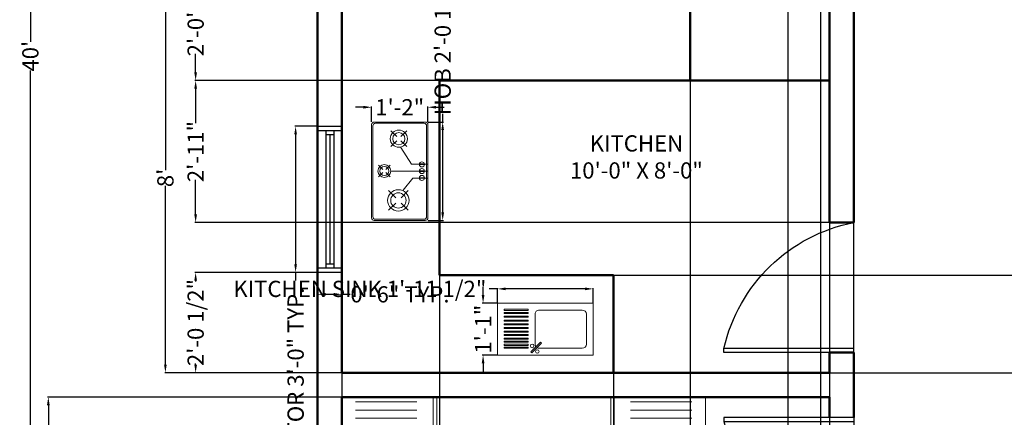
# Model space of a CAD drawing. Units: inches. Extents: x 2663 to 3147, y 140 to 736.
# Tile 2 of 6: x 2663 to 2905, y 327 to 425. Entities that reach past the tile are written whole.
import ezdxf

# ---------------------------------------------------------------- set-up
doc = ezdxf.new("R2010")
doc.units = ezdxf.units.IN
doc.header["$MEASUREMENT"] = 0
for name, color, linetype, lineweight in [('A-ANNO-DIMS', 2, 'Continuous', 18), ('A-AREA-IDEN', 3, 'Continuous', 25), ('A-DOOR', 3, 'Continuous', 25), ('A-FLOR-FIXT', 9, 'Continuous', 18), ('A-FURN', 8, 'Continuous', 18), ('A-GLAZ', 4, 'Continuous', 25), ('A-WALL', 7, 'Continuous', 50)]:
    doc.layers.add(name, color=color, linetype=linetype, lineweight=lineweight)
doc.styles.get("Standard").update_dxf_attribs({"font": 'arial.ttf'})
doc.dimstyles.get("Standard").update_dxf_attribs({"dimtxt": 4, "dimasz": 2, "dimexe": 0.18, "dimexo": 0.0625, "dimgap": 0.09, "dimtad": 0, "dimdec": 0, "dimzin": 0, "dimdsep": 46, "dimlunit": 4, "dimtxsty": 'Standard', "dimcen": 0.09, "dimadec": 0, "dimazin": 0, "dimtfac": 1, "dimtdec": 0, "dimtofl": 0, "dimtmove": 0, "dimatfit": 3, "dimfxl": 1, "dimtolj": 1, "dimtzin": 0, "dimarcsym": 0})

# ---------------------------------------------------------------- blocks, each defined once
blk = doc.blocks.new('*D4')
at = {"layer": 'A-ANNO-DIMS', "color": 0, "lineweight": -2, "transparency": 16777216}
for p, q in [((2742.1, 332.32), (2669.73, 332.32)), ((2669.91, 330.32), (2669.91, 264.1)), ((2669.91, 184.32), (2669.91, 250.55)), ((2742.1, 182.32), (2669.73, 182.32))]:
    blk.add_line(p, q, dxfattribs=at)
at = {"layer": 'A-ANNO-DIMS', "color": 0, "transparency": 16777216}
for points in [[(2669.57, 330.32), (2670.24, 330.32), (2669.91, 332.32)], [(2669.57, 184.32), (2670.24, 184.32), (2669.91, 182.32)]]:
    blk.add_solid(points, dxfattribs=at)
at = {"layer": 'Defpoints', "color": 0, "transparency": 16777216}
for p in [(2669.91, 332.32), (2742.16, 332.32), (2742.16, 182.32)]:
    blk.add_point(p, dxfattribs=at)
at = {"layer": 'A-ANNO-DIMS', "color": 0, "transparency": 16777216, "insert": (2669.91, 257.32), "char_height": 4, "attachment_point": 5, "rotation": 90}
blk.add_mtext('\\A1;12\'-6"', dxfattribs=at)
blk = doc.blocks.new('*D5')
at = {"layer": 'A-ANNO-DIMS', "color": 0, "lineweight": -2, "transparency": 16777216}
for p, q in [((2742.1, 434.32), (2698.54, 434.32)), ((2698.72, 432.32), (2698.72, 388.26)), ((2698.72, 340.32), (2698.72, 384.39)), ((2742.1, 338.32), (2698.54, 338.32))]:
    blk.add_line(p, q, dxfattribs=at)
at = {"layer": 'A-ANNO-DIMS', "color": 0, "transparency": 16777216}
for points in [[(2698.38, 432.32), (2699.05, 432.32), (2698.72, 434.32)], [(2698.38, 340.32), (2699.05, 340.32), (2698.72, 338.32)]]:
    blk.add_solid(points, dxfattribs=at)
at = {"layer": 'Defpoints', "color": 0, "transparency": 16777216}
for p in [(2698.72, 434.32), (2742.16, 434.32), (2742.16, 338.32)]:
    blk.add_point(p, dxfattribs=at)
at = {"layer": 'A-ANNO-DIMS', "color": 0, "transparency": 16777216, "insert": (2698.72, 386.32), "char_height": 4, "attachment_point": 5, "rotation": 90}
blk.add_mtext("\\A1;8'", dxfattribs=at)
blk = doc.blocks.new('FGCHBJK')
for p, q in [((3315.88, 342.07), (3315.88, 348.07)), ((3315.88, 348.07), (3351.88, 348.07)), ((3316.88, 342.07), (3316.88, 348.07)), ((3350.88, 348.07), (3350.88, 342.07)), ((3351.88, 348.07), (3351.88, 342.07)), ((3316.88, 346.07), (3350.88, 346.07)), ((3316.88, 344.07), (3350.88, 344.07)), ((3317.88, 344.07), (3317.88, 346.07)), ((3317.88, 345.07), (3349.88, 345.07)), ((3349.88, 346.07), (3349.88, 344.07)), ((3351.88, 342.07), (3315.88, 342.07))]:
    blk.add_line(p, q)
blk = doc.blocks.new('A$C34930FF8')
at = {"ltscale": 0.05}
for p, q in [((0, 2252.4), (0, 16.8)), ((600, 2252.4), (0, 2252.4)), ((185.4, 1513), (185.4, 1521.5)), ((237.7, 1513), (237.7, 1521.5)), ((227.1, 1479.2), (233.2, 1485.2)), ((436.7, 1513), (436.7, 1504.4)), ((482.5, 1513), (482.5, 1504.4)), ((263.6, 1441.7), (269.7, 1447.7)), ((398.2, 1303.6), (392.1, 1297.6)), ((185.4, 1229.1), (185.4, 1237.7)), ((237.7, 1229.1), (237.7, 1237.7)), ((434.8, 1266.1), (428.7, 1260.1)), ((436.7, 1228.2), (436.7, 1219.7)), ((482.5, 1228.2), (482.5, 1219.7)), ((209.5, 1150.1), (214.1, 1157.3)), ((253.5, 1121.8), (258.1, 1129)), ((415.3, 1017.6), (410.6, 1010.5)), ((459.3, 989.3), (454.7, 982.1)), ((482.5, 894.9), (482.5, 886.3)), ((237.7, 775.3), (237.7, 783.9)), ((436.7, 775.3), (436.7, 766.8)), ((482.5, 775.3), (482.5, 766.8)), ((600, 16.8), (0, 16.8))]:
    blk.add_line(p, q, dxfattribs=at)
for p, q in [((580, 1690.9), (580, 2252.4)), ((600, 1669.3), (600, 2269.3)), ((30, 1790.9), (30, 2169.3)), ((80, 1790.9), (80, 2169.3)), ((130, 1790.9), (130, 2169.3)), ((180, 1790.9), (180, 2169.3)), ((230, 1790.9), (230, 2169.3)), ((280, 1790.9), (280, 2169.3)), ((330, 1790.9), (330, 2169.3)), ((380, 1790.9), (380, 2169.3)), ((430, 1790.9), (430, 2169.3)), ((480, 1790.9), (480, 2169.3)), ((530, 1790.9), (530, 2169.3)), ((580, 1690.9), (0, 1690.9)), ((600, 1669.3), (0, 1669.3)), ((335.4, 1666.1), (335.4, 603.1)), ((600, 1603.3), (620, 1603.3)), ((600, 1018.7), (600, 1603.3)), ((620, 1603.3), (620, 1018.7)), ((237.7, 1521.5), (185.4, 1521.5)), ((482.5, 1513), (185.4, 1513)), ((434.8, 1266.1), (227.4, 1478.9)), ((269.7, 1447.7), (233.2, 1485.2)), ((436.7, 1504.4), (482.5, 1504.4)), ((428.7, 1260.1), (392.1, 1297.6)), ((237.7, 1237.7), (185.4, 1237.7)), ((482.5, 1228.2), (185.4, 1228.2)), ((436.7, 1219.7), (482.5, 1219.7)), ((600, 1233.4), (580, 1233.4)), ((580, 1233.4), (580, 648.7)), ((600, 648.7), (600, 1233.4)), ((258.1, 1129), (214.1, 1157.3)), ((459.3, 989.3), (209.5, 1150.1)), ((454.7, 982.1), (410.6, 1010.5)), ((620, 1018.7), (600, 1018.7)), ((482.5, 894.9), (185.4, 894.9)), ((436.7, 886.3), (482.5, 886.3)), ((237.7, 783.9), (185.4, 783.9)), ((482.5, 775.3), (185.4, 775.3)), ((436.7, 766.8), (482.5, 766.8)), ((580, 648.7), (600, 648.7)), ((600, 600), (0, 600)), ((580, 578.3), (0, 578.3)), ((580, 578.3), (580, 16.8)), ((600, 600), (600, 0)), ((30, 478.3), (30, 100)), ((80, 478.3), (80, 100)), ((130, 478.3), (130, 100)), ((180, 478.3), (180, 100)), ((230, 478.3), (230, 100)), ((280, 478.3), (280, 100)), ((330, 478.3), (330, 100)), ((380, 478.3), (380, 100)), ((430, 478.3), (430, 100)), ((480, 478.3), (480, 100)), ((530, 478.3), (530, 100))]:
    blk.add_line(p, q)
blk = doc.blocks.new('DXFGVHBJKL')
for p, q in [((2908.16, 532.32), (2907.16, 532.32)), ((2907.16, 532.32), (2907.16, 500.32)), ((2908.16, 500.32), (2908.16, 532.32)), ((2908.16, 500.32), (2876.16, 500.32))]:
    blk.add_line(p, q)
blk.add_arc((2916.21, 492.54), 40.8, 102.812, 169.0067)
blk = doc.blocks.new('A$C67F5712B')
for p, q in [((0, 415), (0, 20)), ((10, 405), (10, 30)), ((20, 435), (742, 435)), ((30, 425), (732, 425)), ((336.9, 382.4), (370.3, 349)), ((428.4, 382.4), (394.9, 349)), ((752, 405), (752, 30)), ((762, 415), (762, 20)), ((336.9, 291), (370.3, 324.4)), ((428.4, 291), (394.9, 324.4)), ((79.2, 304.2), (134.9, 248.4)), ((231.6, 304.2), (175.9, 248.4)), ((381, 65.3), (381, 287.1)), ((572, 285.4), (616.6, 240.8)), ((694, 285.4), (649.4, 240.8)), ((79.2, 151.7), (134.9, 207.5)), ((231.6, 151.7), (175.9, 207.5)), ((234.5, 189.9), (328.8, 115.2)), ((435.3, 127.1), (564.3, 209.7)), ((572, 163.4), (616.6, 208)), ((694, 163.4), (649.4, 208)), ((328.8, 65.3), (328.8, 115.2)), ((435.3, 65.3), (435.3, 127.1)), ((30, 10), (732, 10)), ((327.2, 61), (331, 61)), ((327.2, 30.4), (327.2, 61)), ((331, 30.4), (327.2, 30.4)), ((328.8, 0), (328.8, 25.9)), ((331, 61), (331, 30.4)), ((379.4, 61), (383.2, 61)), ((379.4, 30.4), (379.4, 61)), ((383.2, 30.4), (379.4, 30.4)), ((381, 0), (381, 25.9)), ((383.2, 61), (383.2, 30.4)), ((433.7, 61), (437.5, 61)), ((433.7, 30.4), (433.7, 61)), ((437.5, 30.4), (433.7, 30.4)), ((435.3, 0), (435.3, 25.9)), ((437.5, 61), (437.5, 30.4)), ((20, 0), (742, 0))]:
    blk.add_line(p, q)
for centre, radius in [((382.6, 336.7), 49.7), ((155.4, 228), 82.8), ((382.6, 336.7), 35.4), ((155.4, 228), 59), ((633, 224.4), 66.2), ((633, 224.4), 47.2), ((329.2, 45.6), 19.7), ((382.6, 45.6), 19.7), ((434.4, 45.6), 19.7)]:
    blk.add_circle(centre, radius)
for centre, start, end in [((20, 415), 90, 180), ((30, 405), 90, 180), ((732, 405), 0, 90), ((742, 415), 0, 90), ((20, 20), 180, 270), ((30, 30), 180, 270), ((732, 30), 270, 0), ((742, 20), 270, 0)]:
    blk.add_arc(centre, 20, start, end)
blk = doc.blocks.new('A$C49617FB3')
for p, q in [((0, 0), (0, 380.2)), ((0, 380.2), (700.3, 380.2)), ((378.5, 293.7), (448.3, 363.5)), ((448.3, 363.5), (456.5, 355.2)), ((700.3, 380.2), (700.3, 0)), ((50, 80), (50, 300.1)), ((80, 330.1), (395.2, 330.1)), ((386.7, 285.4), (378.5, 293.7)), ((456.5, 355.2), (386.7, 285.4)), ((425.2, 80), (425.2, 300.1)), ((475.2, 322.3), (475.2, 330.1)), ((475.2, 330.1), (650.7, 330.1)), ((475.2, 330.1), (650.3, 330.1)), ((650.7, 322.3), (475.2, 322.3)), ((475.2, 301), (475.2, 308.8)), ((475.2, 308.8), (650.7, 308.8)), ((650.7, 301), (475.2, 301)), ((650.7, 330.1), (650.7, 322.3)), ((650.7, 308.8), (650.7, 301)), ((475.2, 278.2), (475.2, 286)), ((475.2, 286), (650.7, 286)), ((650.7, 278.2), (475.2, 278.2)), ((475.2, 255.4), (475.2, 263.3)), ((475.2, 263.3), (650.7, 263.3)), ((650.7, 255.4), (475.2, 255.4)), ((475.2, 229.8), (475.2, 237.6)), ((475.2, 237.6), (650.7, 237.6)), ((650.7, 229.8), (475.2, 229.8)), ((650.7, 286), (650.7, 278.2)), ((650.7, 263.3), (650.7, 255.4)), ((650.7, 237.6), (650.7, 229.8)), ((475.2, 204.2), (475.2, 212)), ((475.2, 212), (650.7, 212)), ((650.7, 204.2), (475.2, 204.2)), ((475.2, 178.6), (475.2, 186.4)), ((475.2, 186.4), (650.7, 186.4)), ((650.7, 178.6), (475.2, 178.6)), ((475.2, 151.5), (475.2, 159.3)), ((475.2, 159.3), (650.7, 159.3)), ((650.7, 151.5), (475.2, 151.5)), ((650.7, 212), (650.7, 204.2)), ((650.7, 186.4), (650.7, 178.6)), ((650.7, 159.3), (650.7, 151.5)), ((475.2, 124.5), (475.2, 132.3)), ((475.2, 132.3), (650.7, 132.3)), ((650.7, 124.5), (475.2, 124.5)), ((475.2, 94.6), (475.2, 102.4)), ((475.2, 102.4), (650.7, 102.4)), ((650.7, 94.6), (475.2, 94.6)), ((475.2, 67.5), (475.2, 75.4)), ((475.2, 75.4), (650.7, 75.4)), ((650.7, 132.3), (650.7, 124.5)), ((650.7, 102.4), (650.7, 94.6)), ((650.7, 75.4), (650.7, 67.5)), ((395.2, 50), (80, 50)), ((650.7, 67.5), (475.2, 67.5)), ((475.2, 44.8), (475.2, 52.6)), ((475.2, 52.6), (650.7, 52.6)), ((650.7, 44.8), (475.2, 44.8)), ((650.7, 52.6), (650.7, 44.8)), ((700.3, 0), (0, 0))]:
    blk.add_line(p, q)
for centre in [(408.3, 353.3), (446.1, 312.6)]:
    blk.add_circle(centre, 13)
for centre, start, end in [((80, 300.1), 90, 180), ((395.2, 300.1), 58.92551, 90), ((395.2, 300.1), 0, 36.55582), ((80, 80), 180, 270), ((395.2, 80), 270, 0)]:
    blk.add_arc(centre, 30, start, end)
blk = doc.blocks.new('*D37')
at = {"layer": 'A-ANNO-DIMS', "color": 0, "lineweight": -2, "transparency": 16777216}
for p, q in [((2736.1, 656.32), (2665.31, 656.32)), ((2665.49, 654.32), (2665.49, 419.89)), ((2665.49, 178.32), (2665.49, 412.76)), ((2736.1, 176.32), (2665.31, 176.32))]:
    blk.add_line(p, q, dxfattribs=at)
at = {"layer": 'A-ANNO-DIMS', "color": 0, "transparency": 16777216}
for points in [[(2665.15, 654.32), (2665.82, 654.32), (2665.49, 656.32)], [(2665.15, 178.32), (2665.82, 178.32), (2665.49, 176.32)]]:
    blk.add_solid(points, dxfattribs=at)
at = {"layer": 'Defpoints', "color": 0, "transparency": 16777216}
for p in [(2665.49, 656.32), (2736.16, 656.32), (2736.16, 176.32)]:
    blk.add_point(p, dxfattribs=at)
at = {"layer": 'A-ANNO-DIMS', "color": 0, "transparency": 16777216, "insert": (2665.49, 416.32), "char_height": 4, "attachment_point": 5, "rotation": 90}
blk.add_mtext("\\A1;40'", dxfattribs=at)
blk = doc.blocks.new('*D43')
at = {"layer": 'A-ANNO-DIMS', "color": 0, "lineweight": -2, "transparency": 16777216}
for p, q in [((2736.1, 399.04), (2730.58, 399.04)), ((2730.76, 397.04), (2730.76, 365.04)), ((2736.1, 363.04), (2730.58, 363.04)), ((2730.76, 363.04), (2730.76, 361.04))]:
    blk.add_line(p, q, dxfattribs=at)
at = {"layer": 'A-ANNO-DIMS', "color": 0, "transparency": 16777216}
for points in [[(2730.43, 397.04), (2731.09, 397.04), (2730.76, 399.04)], [(2730.43, 365.04), (2731.09, 365.04), (2730.76, 363.04)]]:
    blk.add_solid(points, dxfattribs=at)
at = {"layer": 'Defpoints', "color": 0, "transparency": 16777216}
for p in [(2736.16, 399.04), (2730.76, 363.04), (2736.16, 363.04)]:
    blk.add_point(p, dxfattribs=at)
at = {"layer": 'A-ANNO-DIMS', "color": 0, "transparency": 16777216, "insert": (2730.76, 330.34), "char_height": 4, "attachment_point": 5, "rotation": 90}
blk.add_mtext('\\A1;VENTILATOR 3\'-0" TYP.', dxfattribs=at)
blk = doc.blocks.new('*D44')
at = {"layer": 'A-ANNO-DIMS', "color": 0, "lineweight": -2, "transparency": 16777216}
for p, q in [((2736.16, 362.98), (2736.16, 357.46)), ((2742.16, 362.98), (2742.16, 357.46)), ((2738.16, 357.64), (2740.16, 357.64)), ((2742.16, 357.64), (2744.16, 357.64))]:
    blk.add_line(p, q, dxfattribs=at)
at = {"layer": 'A-ANNO-DIMS', "color": 0, "transparency": 16777216}
for points in [[(2738.16, 357.98), (2738.16, 357.31), (2736.16, 357.64)], [(2740.16, 357.98), (2740.16, 357.31), (2742.16, 357.64)]]:
    blk.add_solid(points, dxfattribs=at)
at = {"layer": 'Defpoints', "color": 0, "transparency": 16777216}
for p in [(2736.16, 363.04), (2742.16, 363.04), (2742.16, 357.64)]:
    blk.add_point(p, dxfattribs=at)
at = {"layer": 'A-ANNO-DIMS', "color": 0, "transparency": 16777216, "insert": (2756.44, 357.64), "char_height": 4, "attachment_point": 5}
blk.add_mtext('\\A1;0\'-6" TYP.', dxfattribs=at)
blk = doc.blocks.new('*D53')
at = {"layer": 'A-ANNO-DIMS', "color": 0, "lineweight": -2, "transparency": 16777216}
for p, q in [((2763.37, 400.1), (2767.13, 400.1)), ((2766.95, 400.1), (2766.95, 402.1)), ((2766.95, 377.83), (2766.95, 398.1)), ((2763.37, 375.83), (2767.13, 375.83))]:
    blk.add_line(p, q, dxfattribs=at)
at = {"layer": 'A-ANNO-DIMS', "color": 0, "transparency": 16777216}
for points in [[(2766.62, 398.1), (2767.29, 398.1), (2766.95, 400.1)], [(2766.62, 377.83), (2767.29, 377.83), (2766.95, 375.83)]]:
    blk.add_solid(points, dxfattribs=at)
at = {"layer": 'Defpoints', "color": 0, "transparency": 16777216}
for p in [(2763.31, 400.1), (2766.95, 400.1), (2763.31, 375.83)]:
    blk.add_point(p, dxfattribs=at)
at = {"layer": 'A-ANNO-DIMS', "color": 0, "transparency": 16777216, "insert": (2766.95, 418.89), "char_height": 4, "attachment_point": 5, "rotation": 90}
blk.add_mtext('\\A1;HOB 2\'-0 1/2"', dxfattribs=at)
blk = doc.blocks.new('*D54')
at = {"layer": 'A-ANNO-DIMS', "color": 0, "lineweight": -2, "transparency": 16777216}
for p, q in [((2747.46, 403.74), (2745.46, 403.74)), ((2749.46, 400.17), (2749.46, 403.92)), ((2763.31, 400.17), (2763.31, 403.92)), ((2765.31, 403.74), (2767.31, 403.74))]:
    blk.add_line(p, q, dxfattribs=at)
at = {"layer": 'A-ANNO-DIMS', "color": 0, "transparency": 16777216}
for points in [[(2747.46, 404.08), (2747.46, 403.41), (2749.46, 403.74)], [(2765.31, 404.08), (2765.31, 403.41), (2763.31, 403.74)]]:
    blk.add_solid(points, dxfattribs=at)
at = {"layer": 'Defpoints', "color": 0, "transparency": 16777216}
for p in [(2749.46, 403.74), (2749.46, 400.1), (2763.31, 400.1)]:
    blk.add_point(p, dxfattribs=at)
at = {"layer": 'A-ANNO-DIMS', "color": 0, "transparency": 16777216, "insert": (2756.38, 403.74), "char_height": 4, "attachment_point": 5}
blk.add_mtext('\\A1;1\'-2"', dxfattribs=at)
blk = doc.blocks.new('*D55')
at = {"layer": 'A-ANNO-DIMS', "color": 0, "lineweight": -2, "transparency": 16777216}
for p, q in [((2780.43, 358.98), (2778.43, 358.98)), ((2780.43, 355.51), (2780.43, 359.16)), ((2802, 358.98), (2782.43, 358.98)), ((2804, 355.51), (2804, 359.16))]:
    blk.add_line(p, q, dxfattribs=at)
at = {"layer": 'A-ANNO-DIMS', "color": 0, "transparency": 16777216}
for points in [[(2782.43, 359.32), (2782.43, 358.65), (2780.43, 358.98)], [(2802, 359.32), (2802, 358.65), (2804, 358.98)]]:
    blk.add_solid(points, dxfattribs=at)
at = {"layer": 'Defpoints', "color": 0, "transparency": 16777216}
for p in [(2780.43, 358.98), (2780.43, 355.45), (2804, 355.45)]:
    blk.add_point(p, dxfattribs=at)
at = {"layer": 'A-ANNO-DIMS', "color": 0, "transparency": 16777216, "insert": (2746.56, 358.98), "char_height": 4, "attachment_point": 5}
blk.add_mtext('\\A1;KITCHEN SINK 1\'-11 1/2"', dxfattribs=at)
blk = doc.blocks.new('*D56')
at = {"layer": 'A-ANNO-DIMS', "color": 0, "lineweight": -2, "transparency": 16777216}
for p, q in [((2776.89, 357.45), (2776.89, 359.45)), ((2780.36, 355.45), (2776.71, 355.45)), ((2780.36, 342.65), (2776.71, 342.65)), ((2776.89, 340.65), (2776.89, 338.65))]:
    blk.add_line(p, q, dxfattribs=at)
at = {"layer": 'A-ANNO-DIMS', "color": 0, "transparency": 16777216}
for points in [[(2776.56, 357.45), (2777.22, 357.45), (2776.89, 355.45)], [(2776.56, 340.65), (2777.22, 340.65), (2776.89, 342.65)]]:
    blk.add_solid(points, dxfattribs=at)
at = {"layer": 'Defpoints', "color": 0, "transparency": 16777216}
for p in [(2780.43, 355.45), (2776.89, 342.65), (2780.43, 342.65)]:
    blk.add_point(p, dxfattribs=at)
at = {"layer": 'A-ANNO-DIMS', "color": 0, "transparency": 16777216, "insert": (2776.89, 349.05), "char_height": 4, "attachment_point": 5, "rotation": 90}
blk.add_mtext('\\A1;1\'-1"', dxfattribs=at)
blk = doc.blocks.new('*D61')
at = {"layer": 'A-ANNO-DIMS', "color": 0, "lineweight": -2, "transparency": 16777216}
for p, q in [((2851.95, 276.84), (2851.95, 686.5)), ((2853.95, 686.32), (2857.98, 686.32)), ((2859.98, 276.84), (2859.98, 686.5)), ((2859.98, 686.32), (2861.98, 686.32))]:
    blk.add_line(p, q, dxfattribs=at)
at = {"layer": 'A-ANNO-DIMS', "color": 0, "transparency": 16777216}
for points in [[(2853.95, 686.66), (2853.95, 685.99), (2851.95, 686.32)], [(2857.98, 686.66), (2857.98, 685.99), (2859.98, 686.32)]]:
    blk.add_solid(points, dxfattribs=at)
at = {"layer": 'Defpoints', "color": 0, "transparency": 16777216}
for p in [(2859.98, 686.32), (2851.95, 276.78), (2859.98, 276.78)]:
    blk.add_point(p, dxfattribs=at)
at = {"layer": 'A-ANNO-DIMS', "color": 0, "transparency": 16777216, "insert": (2867.39, 686.32), "char_height": 4, "attachment_point": 5}
blk.add_mtext('\\A1;0\'-8"', dxfattribs=at)
blk = doc.blocks.new('*D73')
at = {"layer": 'A-ANNO-DIMS', "color": 0, "lineweight": -2, "transparency": 16777216}
for p, q in [((2742.1, 363.04), (2705.98, 363.04)), ((2706.16, 361.04), (2706.16, 360.78)), ((2706.16, 340.32), (2706.16, 340.58)), ((2742.1, 338.32), (2705.98, 338.32))]:
    blk.add_line(p, q, dxfattribs=at)
at = {"layer": 'A-ANNO-DIMS', "color": 0, "transparency": 16777216}
for points in [[(2705.83, 361.04), (2706.49, 361.04), (2706.16, 363.04)], [(2705.83, 340.32), (2706.49, 340.32), (2706.16, 338.32)]]:
    blk.add_solid(points, dxfattribs=at)
at = {"layer": 'Defpoints', "color": 0, "transparency": 16777216}
for p in [(2706.16, 363.04), (2742.16, 363.04), (2742.16, 338.32)]:
    blk.add_point(p, dxfattribs=at)
at = {"layer": 'A-ANNO-DIMS', "color": 0, "transparency": 16777216, "insert": (2706.16, 350.68), "char_height": 4, "attachment_point": 5, "rotation": 90}
blk.add_mtext('\\A1;2\'-0 1/2"', dxfattribs=at)
blk = doc.blocks.new('*D79')
at = {"layer": 'A-ANNO-DIMS', "color": 0, "lineweight": -2, "transparency": 16777216}
for p, q in [((2862.1, 410.32), (2705.98, 410.32)), ((2706.16, 408.32), (2706.16, 399.82)), ((2706.16, 377.32), (2706.16, 385.83)), ((2862.1, 375.32), (2705.98, 375.32))]:
    blk.add_line(p, q, dxfattribs=at)
at = {"layer": 'A-ANNO-DIMS', "color": 0, "transparency": 16777216}
for points in [[(2705.83, 408.32), (2706.49, 408.32), (2706.16, 410.32)], [(2705.83, 377.32), (2706.49, 377.32), (2706.16, 375.32)]]:
    blk.add_solid(points, dxfattribs=at)
at = {"layer": 'Defpoints', "color": 0, "transparency": 16777216}
for p in [(2706.16, 410.32), (2862.16, 410.32), (2862.16, 375.32)]:
    blk.add_point(p, dxfattribs=at)
at = {"layer": 'A-ANNO-DIMS', "color": 0, "transparency": 16777216, "insert": (2706.16, 392.82), "char_height": 4, "attachment_point": 5, "rotation": 90}
blk.add_mtext('\\A1;2\'-11"', dxfattribs=at)
blk = doc.blocks.new('*D80')
at = {"layer": 'A-ANNO-DIMS', "color": 0, "lineweight": -2, "transparency": 16777216}
for p, q in [((2862.1, 434.32), (2705.98, 434.32)), ((2706.16, 432.32), (2706.16, 427.76)), ((2706.16, 412.32), (2706.16, 416.88)), ((2862.1, 410.32), (2705.98, 410.32))]:
    blk.add_line(p, q, dxfattribs=at)
at = {"layer": 'A-ANNO-DIMS', "color": 0, "transparency": 16777216}
for points in [[(2705.83, 432.32), (2706.49, 432.32), (2706.16, 434.32)], [(2705.83, 412.32), (2706.49, 412.32), (2706.16, 410.32)]]:
    blk.add_solid(points, dxfattribs=at)
at = {"layer": 'Defpoints', "color": 0, "transparency": 16777216}
for p in [(2706.16, 434.32), (2862.16, 434.32), (2862.16, 410.32)]:
    blk.add_point(p, dxfattribs=at)
at = {"layer": 'A-ANNO-DIMS', "color": 0, "transparency": 16777216, "insert": (2706.16, 422.32), "char_height": 4, "attachment_point": 5, "rotation": 90}
blk.add_mtext('\\A1;2\'-0"', dxfattribs=at)
blk = doc.blocks.new('*D81')
at = {"layer": 'A-ANNO-DIMS', "color": 0, "lineweight": -2, "transparency": 16777216}
for p, q in [((2827.83, 410.26), (2827.83, 146.14)), ((2862.16, 410.26), (2862.16, 146.14)), ((2829.83, 146.32), (2833.34, 146.32)), ((2860.16, 146.32), (2856.65, 146.32))]:
    blk.add_line(p, q, dxfattribs=at)
at = {"layer": 'A-ANNO-DIMS', "color": 0, "transparency": 16777216}
for points in [[(2829.83, 146.66), (2829.83, 145.99), (2827.83, 146.32)], [(2860.16, 146.66), (2860.16, 145.99), (2862.16, 146.32)]]:
    blk.add_solid(points, dxfattribs=at)
at = {"layer": 'Defpoints', "color": 0, "transparency": 16777216}
for p in [(2827.83, 410.32), (2862.16, 410.32), (2862.16, 146.32)]:
    blk.add_point(p, dxfattribs=at)
at = {"layer": 'A-ANNO-DIMS', "color": 0, "transparency": 16777216, "insert": (2845, 146.32), "char_height": 4, "attachment_point": 5}
blk.add_mtext('\\A1;2\'-10 1/2"', dxfattribs=at)
blk = doc.blocks.new('*D82')
at = {"layer": 'A-ANNO-DIMS', "color": 0, "lineweight": -2, "transparency": 16777216}
for p, q in [((2742.16, 362.98), (2742.16, 146.14)), ((2766.16, 362.26), (2766.16, 146.14)), ((2744.16, 146.32), (2748.72, 146.32)), ((2764.16, 146.32), (2759.6, 146.32))]:
    blk.add_line(p, q, dxfattribs=at)
at = {"layer": 'A-ANNO-DIMS', "color": 0, "transparency": 16777216}
for points in [[(2744.16, 146.66), (2744.16, 145.99), (2742.16, 146.32)], [(2764.16, 146.66), (2764.16, 145.99), (2766.16, 146.32)]]:
    blk.add_solid(points, dxfattribs=at)
at = {"layer": 'Defpoints', "color": 0, "transparency": 16777216}
for p in [(2742.16, 363.04), (2766.16, 362.32), (2766.16, 146.32)]:
    blk.add_point(p, dxfattribs=at)
at = {"layer": 'A-ANNO-DIMS', "color": 0, "transparency": 16777216, "insert": (2754.16, 146.32), "char_height": 4, "attachment_point": 5}
blk.add_mtext('\\A1;2\'-0"', dxfattribs=at)
blk = doc.blocks.new('*D83')
at = {"layer": 'A-ANNO-DIMS', "color": 0, "lineweight": -2, "transparency": 16777216}
for p, q in [((2766.16, 362.26), (2766.16, 146.14)), ((2808.99, 362.26), (2808.99, 146.14)), ((2768.16, 146.32), (2782.17, 146.32)), ((2806.99, 146.32), (2792.98, 146.32))]:
    blk.add_line(p, q, dxfattribs=at)
at = {"layer": 'A-ANNO-DIMS', "color": 0, "transparency": 16777216}
for points in [[(2768.16, 146.66), (2768.16, 145.99), (2766.16, 146.32)], [(2806.99, 146.66), (2806.99, 145.99), (2808.99, 146.32)]]:
    blk.add_solid(points, dxfattribs=at)
at = {"layer": 'Defpoints', "color": 0, "transparency": 16777216}
for p in [(2766.16, 362.32), (2808.99, 362.32), (2808.99, 146.32)]:
    blk.add_point(p, dxfattribs=at)
at = {"layer": 'A-ANNO-DIMS', "color": 0, "transparency": 16777216, "insert": (2787.58, 146.32), "char_height": 4, "attachment_point": 5}
blk.add_mtext('\\A1;3\'-7"', dxfattribs=at)
blk = doc.blocks.new('*D84')
at = {"layer": 'A-ANNO-DIMS', "color": 0, "lineweight": -2, "transparency": 16777216}
for p, q in [((2809.05, 362.32), (3126.34, 362.32)), ((3126.16, 360.32), (3126.16, 355.76)), ((3126.16, 340.32), (3126.16, 344.88)), ((2809.05, 338.32), (3126.34, 338.32))]:
    blk.add_line(p, q, dxfattribs=at)
at = {"layer": 'A-ANNO-DIMS', "color": 0, "transparency": 16777216}
for points in [[(3125.83, 360.32), (3126.49, 360.32), (3126.16, 362.32)], [(3125.83, 340.32), (3126.49, 340.32), (3126.16, 338.32)]]:
    blk.add_solid(points, dxfattribs=at)
at = {"layer": 'Defpoints', "color": 0, "transparency": 16777216}
for p in [(2808.99, 362.32), (3126.16, 362.32), (2808.99, 338.32)]:
    blk.add_point(p, dxfattribs=at)
at = {"layer": 'A-ANNO-DIMS', "color": 0, "transparency": 16777216, "insert": (3126.16, 350.32), "char_height": 4, "attachment_point": 5, "rotation": 90}
blk.add_mtext('\\A1;2\'-0"', dxfattribs=at)

msp = doc.modelspace()

# ---------------------------------------------------------------- linework, layer by layer
at = {"layer": 'A-WALL'}
for p, q in [((2736.16, 176.32), (2736.16, 656.32)), ((2868.16, 375.32), (2868.16, 440.32)), ((2742.16, 338.32), (2742.16, 434.32)), ((2827.83, 434.32), (2827.83, 410.32)), ((2862.16, 375.32), (2862.16, 434.32)), ((2766.16, 362.32), (2766.16, 410.32)), ((2766.16, 410.32), (2862.16, 410.32)), ((2862.16, 375.32), (2868.16, 375.32)), ((2766.16, 362.32), (2808.99, 362.32)), ((2808.99, 362.32), (2808.99, 338.32)), ((2862.16, 338.32), (2862.16, 343.32)), ((2862.16, 343.32), (2868.16, 343.32)), ((2868.16, 327.32), (2868.16, 343.32)), ((2742.16, 338.32), (2862.16, 338.32)), ((2742.16, 182.32), (2742.16, 332.32)), ((2742.16, 332.32), (2862.16, 332.32)), ((2862.16, 327.32), (2862.16, 332.32))]:
    msp.add_line(p, q, dxfattribs=at)

# ---------------------------------------------------------------- block references
at = {"layer": 'A-DOOR', "xscale": -1, "rotation": 90}
msp.add_blockref('DXFGVHBJKL', (3368.49, 3251.49), dxfattribs=at)
at = {"layer": 'A-DOOR', "rotation": 90.00000000000003}
msp.add_blockref('DXFGVHBJKL', (3368.49, -2580.84), dxfattribs=at)
at = {"layer": 'A-FLOR-FIXT'}
for name, p, xscale, yscale, zscale, rotation in [('A$C67F5712B', (2763.31, 375.83), 0.0318512609147648, 0.0318512609147648, 0.0318512609147648, 90), ('A$C49617FB3', (2804, 355.45), 0.0336566378947754, 0.0336566378947754, 0.0336566378947754, 180)]:
    msp.add_blockref(name, p, dxfattribs=dict(at, xscale=xscale, yscale=yscale, zscale=zscale, rotation=rotation))
at = {"layer": 'A-FURN', "xscale": 0.0400188077054237, "yscale": 0.0400188077054237, "zscale": 0.0400188077054237, "rotation": 270}
msp.add_blockref('A$C34930FF8', (2741.49, 332.32), dxfattribs=at)
at = {"layer": 'A-GLAZ', "rotation": 270}
msp.add_blockref('FGCHBJK', (2394.09, 3714.93), dxfattribs=at)

# ---------------------------------------------------------------- texts
at = {"layer": 'A-AREA-IDEN', "insert": (2776.13, 396.83), "char_height": 4, "attachment_point": 1}
msp.add_mtext_dynamic_manual_height_columns('\\pxqc;KITCHEN\\P10\'-0" X 8\'-0"', width=76.9916, gutter_width=20, heights=[0], dxfattribs=at)

# ---------------------------------------------------------------- dimensions: what is measured, and where the dimension line sits
at = {"layer": 'A-ANNO-DIMS'}
for base, p1, p2, picture, middle in [((2859.98, 686.32), (2851.95, 276.78), (2859.98, 276.78), '*D61', (2867.39, 686.32)), ((2862.16, 146.32), (2827.83, 410.32), (2862.16, 410.32), '*D81', (2845, 146.32)), ((2766.16, 146.32), (2742.16, 363.04), (2766.16, 362.32), '*D82', (2754.16, 146.32)), ((2808.99, 146.32), (2766.16, 362.32), (2808.99, 362.32), '*D83', (2787.58, 146.32))]:
    dim = msp.add_linear_dim(base=base, p1=p1, p2=p2, dimstyle='Standard', override={"dimdec": 1, "dimlfac": 1, "dimrnd": 0, "dimzin": 1, "dimdsep": 46, "dimlunit": 4, "dimfrac": 2}, dxfattribs=at)
    dim.commit()
    dim.dimension.update_dxf_attribs({"geometry": picture, "text_midpoint": middle})
for base, p1, p2, angle, override, picture, middle in [((2665.49, 656.32), (2736.16, 176.32), (2736.16, 656.32), 90, {"dimclrd": 0, "dimclre": 0, "dimclrt": 0}, '*D37', (2665.49, 416.32)), ((2698.72, 434.32), (2742.16, 338.32), (2742.16, 434.32), 90, {"dimclrd": 0, "dimclre": 0, "dimclrt": 0}, '*D5', (2698.72, 386.32)), ((2706.16, 434.32), (2862.16, 410.32), (2862.16, 434.32), 90, {"dimdec": 1, "dimlfac": 1, "dimrnd": 0, "dimzin": 1, "dimdsep": 46, "dimlunit": 4, "dimfrac": 2}, '*D80', (2706.16, 422.32)), ((2706.16, 410.32), (2862.16, 375.32), (2862.16, 410.32), 90, {"dimdec": 1, "dimlfac": 1, "dimrnd": 0, "dimzin": 1, "dimdsep": 46, "dimlunit": 4, "dimfrac": 2}, '*D79', (2706.16, 392.82)), ((2749.4563, 403.7445), (2763.3116, 400.1039), (2749.4563, 400.1039), 180, {"dimdec": 1, "dimrnd": 0, "dimzin": 1, "dimlunit": 4, "dimfrac": 2}, '*D54', (2756.3839, 403.7445)), ((2706.16, 363.04), (2742.16, 338.32), (2742.16, 363.04), 90, {"dimdec": 1, "dimlfac": 1, "dimrnd": 0, "dimzin": 1, "dimdsep": 46, "dimlunit": 4, "dimfrac": 2}, '*D73', (2706.16, 350.68)), ((3126.16, 362.32), (2808.99, 338.32), (2808.99, 362.32), 90, {"dimdec": 1, "dimlfac": 1, "dimrnd": 0, "dimzin": 1, "dimdsep": 46, "dimlunit": 4, "dimfrac": 2}, '*D84', (3126.16, 350.32)), ((2776.89, 342.65), (2780.43, 355.45), (2780.43, 342.65), 270, {"dimdec": 1, "dimrnd": 0, "dimzin": 1, "dimlunit": 4, "dimfrac": 2}, '*D56', (2776.89, 349.05)), ((2669.91, 332.32), (2742.16, 182.32), (2742.16, 332.32), 90, {"dimclrd": 0, "dimclre": 0, "dimclrt": 0}, '*D4', (2669.91, 257.32))]:
    dim = msp.add_linear_dim(base=base, p1=p1, p2=p2, angle=angle, dimstyle='Standard', override=override, dxfattribs=at)
    dim.commit()
    dim.dimension.update_dxf_attribs({"geometry": picture, "text_midpoint": middle})
for base, p1, p2, angle, text, picture, middle in [((2766.95, 400.1), (2763.31, 375.83), (2763.31, 400.1), 90, 'HOB <>', '*D53', (2766.95, 418.89)), ((2730.76, 363.04), (2736.16, 399.04), (2736.16, 363.04), 270, 'VENTILATOR <> TYP.', '*D43', (2730.76, 330.34)), ((2780.43, 358.98), (2804, 355.45), (2780.43, 355.45), 180, 'KITCHEN SINK <>', '*D55', (2746.56, 358.98))]:
    dim = msp.add_linear_dim(base=base, p1=p1, p2=p2, angle=angle, text=text, dimstyle='Standard', override={"dimdec": 1, "dimrnd": 0, "dimzin": 1, "dimlunit": 4, "dimfrac": 2}, dxfattribs=at)
    dim.commit()
    dim.dimension.update_dxf_attribs({"geometry": picture, "text_midpoint": middle})
dim = msp.add_linear_dim(base=(2742.16, 357.64), p1=(2736.16, 363.04), p2=(2742.16, 363.04), text='<> TYP.', dimstyle='Standard', override={"dimdec": 1, "dimrnd": 0, "dimzin": 1, "dimlunit": 4, "dimfrac": 2}, dxfattribs=at)
dim.commit()
dim.dimension.update_dxf_attribs({"geometry": '*D44', "text_midpoint": (2756.44, 357.64)})

doc.saveas('drawing.dxf')
